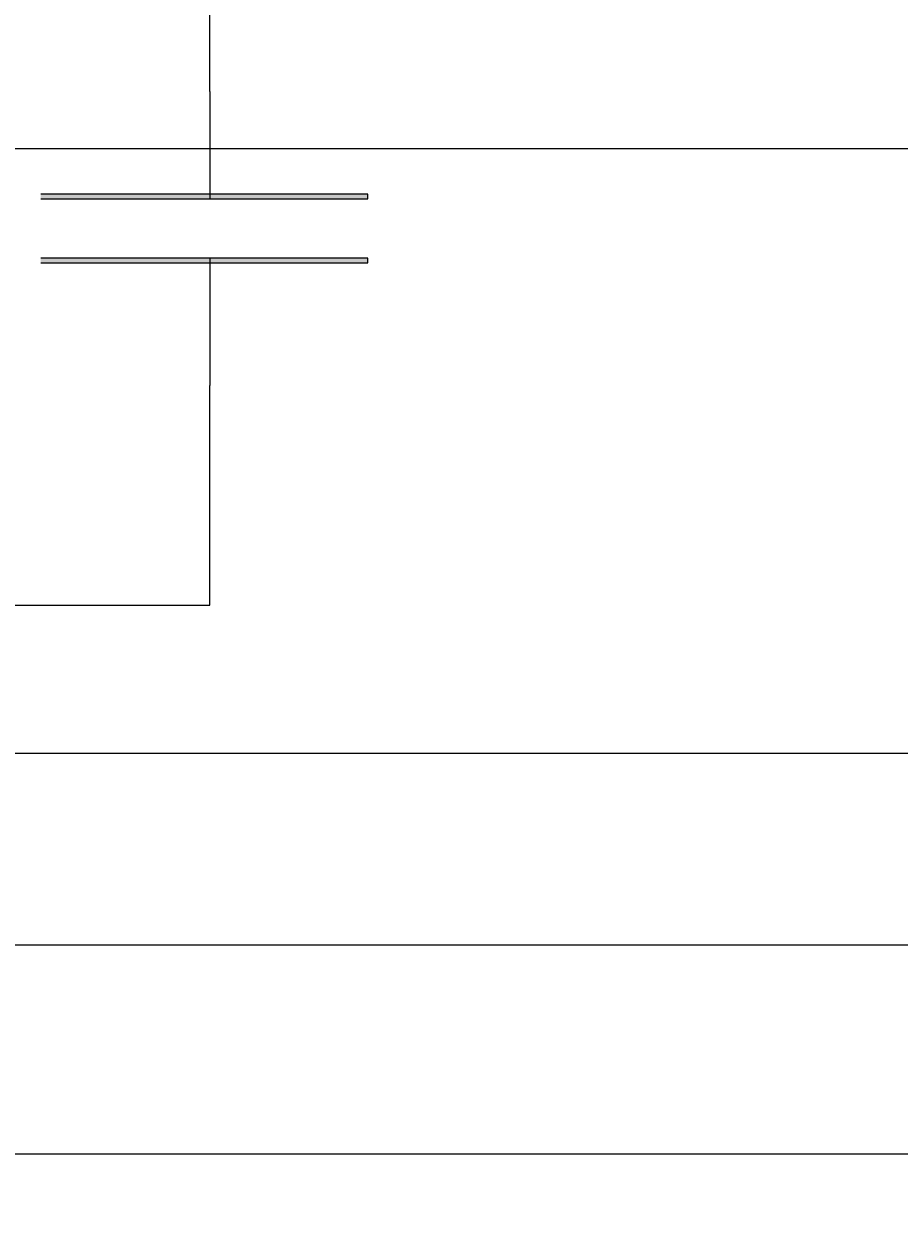
# Model space of a CAD drawing. Units: inches. Extents: x 35362 to 73946, y 43607 to 67532.
# Tile 134 of 134: x 69277 to 71350, y 55752 to 58575. Entities that reach past the tile are written whole.
import ezdxf

# ---------------------------------------------------------------- set-up
doc = ezdxf.new("R2010")
doc.units = ezdxf.units.IN
doc.header["$MEASUREMENT"] = 0
for name, color, linetype, lineweight in [('A-ANNO-DIMS', 2, 'Continuous', 18), ('E-SYMB', 1, 'Continuous', 25), ('E-SYMB-PATT', 1, 'Continuous', 13), ('E-WIRE', 3, 'Continuous', 25)]:
    doc.layers.add(name, color=color, linetype=linetype, lineweight=lineweight)
doc.styles.get("Standard").update_dxf_attribs({"font": 'arial.ttf'})
doc.dimstyles.get("Standard").update_dxf_attribs({"dimtxt": 0.18, "dimasz": 0.18, "dimexe": 0.18, "dimexo": 0.0625, "dimgap": 0.09, "dimtad": 0, "dimtih": 1, "dimtoh": 1, "dimdec": 4, "dimzin": 0, "dimdsep": 46, "dimtxsty": 'Standard', "dimcen": 0.09, "dimadec": 0, "dimazin": 0, "dimtfac": 1, "dimtdec": 4, "dimtofl": 0, "dimtmove": 0, "dimatfit": 3, "dimfxl": 1, "dimtolj": 1, "dimtzin": 0, "dimarcsym": 0})

# ---------------------------------------------------------------- blocks, each defined once
blk = doc.blocks.new('*D8')
at = {"layer": 'A-ANNO-DIMS', "color": 0, "lineweight": -2, "transparency": 16777216}
for p, q in [((66271.28651900003, 65771.51172800003), (73945.82566600003, 65771.51172800003)), ((73945.64566600005, 65771.33172800003), (73945.64566600005, 59737.03093663782)), ((73945.64566600005, 53702.36633900002), (73945.64566600005, 59736.66713036224)), ((72185.70816600003, 53702.18633900003), (73945.82566600003, 53702.18633900003))]:
    blk.add_line(p, q, dxfattribs=at)
at = {"layer": 'A-ANNO-DIMS', "color": 0, "transparency": 16777216}
for points in [[(73945.61566600006, 65771.33172800003), (73945.67566600005, 65771.33172800003), (73945.64566600005, 65771.51172800003)], [(73945.61566600006, 53702.36633900002), (73945.67566600005, 53702.36633900002), (73945.64566600005, 53702.18633900003)]]:
    blk.add_solid(points, dxfattribs=at)
at = {"layer": 'Defpoints', "color": 0, "transparency": 16777216}
for p in [(66271.22401900003, 65771.51172800003), (73945.64566600005, 65771.51172800003), (72185.64566600003, 53702.18633900003)]:
    blk.add_point(p, dxfattribs=at)
at = {"layer": 'A-ANNO-DIMS', "color": 0, "transparency": 16777216, "insert": (73945.64566600005, 59736.84903349999), "char_height": 0.18, "attachment_point": 5}
blk.add_mtext('\\A1;12069', dxfattribs=at)
blk = doc.blocks.new('*D10')
at = {"layer": 'A-ANNO-DIMS', "color": 0, "lineweight": -2, "transparency": 16777216}
for p, q in [((61240.96983600002, 59185.14395700003), (73945.82566600003, 59185.14395700003)), ((73945.64566600005, 59184.96395700003), (73945.64566600005, 56268.51827402935)), ((73945.64566600005, 53351.70866200003), (73945.64566600005, 56268.1543449707)), ((61240.96983600002, 53351.52866200003), (73945.82566600003, 53351.52866200003))]:
    blk.add_line(p, q, dxfattribs=at)
at = {"layer": 'A-ANNO-DIMS', "color": 0, "transparency": 16777216}
for points in [[(73945.61566600006, 59184.96395700003), (73945.67566600005, 59184.96395700003), (73945.64566600005, 59185.14395700003)], [(73945.61566600006, 53351.70866200003), (73945.67566600005, 53351.70866200003), (73945.64566600005, 53351.52866200003)]]:
    blk.add_solid(points, dxfattribs=at)
at = {"layer": 'Defpoints', "color": 0, "transparency": 16777216}
for p in [(61240.90733600002, 59185.14395700003), (61240.90733600002, 53351.52866200003), (73945.64566600005, 53351.52866200003)]:
    blk.add_point(p, dxfattribs=at)
at = {"layer": 'A-ANNO-DIMS', "color": 0, "transparency": 16777216, "insert": (73945.64566600005, 56268.33630949999), "char_height": 0.18, "attachment_point": 5}
blk.add_mtext('\\A1;5834', dxfattribs=at)
blk = doc.blocks.new('*D47')
at = {"layer": 'A-ANNO-DIMS', "color": 0, "lineweight": -2, "transparency": 16777216}
for p, q in [((50339.58680000003, 58279.98849500002), (73945.82566600003, 58279.98849500002)), ((73945.64566600005, 58279.80849500002), (73945.64566600005, 57564.17141502935)), ((73945.64566600005, 56848.17040600003), (73945.64566600005, 57563.80748597069)), ((50339.58680000003, 56847.99040600003), (73945.82566600003, 56847.99040600003))]:
    blk.add_line(p, q, dxfattribs=at)
at = {"layer": 'A-ANNO-DIMS', "color": 0, "transparency": 16777216}
for points in [[(73945.61566600006, 58279.80849500002), (73945.67566600005, 58279.80849500002), (73945.64566600005, 58279.98849500002)], [(73945.61566600006, 56848.17040600003), (73945.67566600005, 56848.17040600003), (73945.64566600005, 56847.99040600003)]]:
    blk.add_solid(points, dxfattribs=at)
at = {"layer": 'Defpoints', "color": 0, "transparency": 16777216}
for p in [(50339.52430000002, 58279.98849500002), (50339.52430000002, 56847.99040600003), (73945.64566600005, 56847.99040600003)]:
    blk.add_point(p, dxfattribs=at)
at = {"layer": 'A-ANNO-DIMS', "color": 0, "transparency": 16777216, "insert": (73945.64566600005, 57563.98945049999), "char_height": 0.18, "attachment_point": 5}
blk.add_mtext('\\A1;1432.0', dxfattribs=at)
blk = doc.blocks.new('*D50')
at = {"layer": 'A-ANNO-DIMS', "color": 0, "lineweight": -2, "transparency": 16777216}
for p, q in [((61657.28213900003, 56394.41825000003), (73945.82566600003, 56394.41825000003)), ((73945.64566600005, 56394.23825000003), (73945.64566600005, 56147.19337413782)), ((73945.64566600005, 55899.78469200003), (73945.64566600005, 56146.82956786224)), ((61657.28213900003, 55899.60469200002), (73945.82566600003, 55899.60469200002))]:
    blk.add_line(p, q, dxfattribs=at)
at = {"layer": 'A-ANNO-DIMS', "color": 0, "transparency": 16777216}
for points in [[(73945.61566600006, 56394.23825000003), (73945.67566600005, 56394.23825000003), (73945.64566600005, 56394.41825000003)], [(73945.61566600006, 55899.78469200003), (73945.67566600005, 55899.78469200003), (73945.64566600005, 55899.60469200002)]]:
    blk.add_solid(points, dxfattribs=at)
at = {"layer": 'Defpoints', "color": 0, "transparency": 16777216}
for p in [(61657.21963900003, 56394.41825000003), (61657.21963900003, 55899.60469200002), (73945.64566600005, 55899.60469200002)]:
    blk.add_point(p, dxfattribs=at)
at = {"layer": 'A-ANNO-DIMS', "color": 0, "transparency": 16777216, "insert": (73945.64566600005, 56147.01147099999), "char_height": 0.18, "attachment_point": 5}
blk.add_mtext('\\A1;494.8', dxfattribs=at)

msp = doc.modelspace()

# ---------------------------------------------------------------- hatches: boundary and pattern name
at = {"layer": 'E-SYMB-PATT'}
h = msp.add_hatch(color=256, dxfattribs=at)
h.dxf.hatch_style = 1
h.paths.add_polyline_path([(70091.40622432147, 58160.31058347617), (70091.40622432147, 58171.46529320917), (69317.27150299007, 58171.46529320917), (69317.27150299007, 58160.31058347618)])
h = msp.add_hatch(color=256, dxfattribs=at)
h.dxf.hatch_style = 1
h.paths.add_polyline_path([(70091.40622432147, 58009.34910605), (70091.40622432147, 58020.50381578299), (69317.27150299007, 58020.50381578299), (69317.27150299007, 58009.34910605)])

# ---------------------------------------------------------------- linework, layer by layer
at = {"layer": 'E-SYMB'}
for p, q in [((69717.45127656072, 58414.54422497431), (69717.45127656074, 58160.31058347618)), ((70091.40622432147, 58171.46529320917), (69317.27150299007, 58171.46529320917)), ((69317.27150299007, 58160.31058347618), (70091.40622432147, 58160.31058347617)), ((70091.40622432147, 58160.31058347617), (70091.40622432147, 58171.46529320917)), ((70091.40622432147, 58020.50381578299), (69317.27150299007, 58020.50381578299)), ((69717.45127656074, 58020.50381578299), (69717.45127656072, 57718.9486764754)), ((70091.40622432147, 58009.34910605), (70091.40622432147, 58020.50381578299)), ((69317.27150299007, 58009.34910605), (70091.40622432147, 58009.34910605))]:
    msp.add_line(p, q, dxfattribs=at)
at = {"layer": 'E-WIRE'}
for p, q in [((69717.45127656072, 58414.54422497431), (69717.45127656072, 58648.13900443873)), ((69717.45127656069, 57198.49827444748), (69717.45127656072, 57718.9486764754)), ((68678.61631230469, 57198.49827444747), (69717.45127656069, 57198.49827444748))]:
    msp.add_line(p, q, dxfattribs=at)

# ---------------------------------------------------------------- dimensions: what is measured, and where the dimension line sits
at = {"layer": 'A-ANNO-DIMS'}
for base, p1, p2, override, picture, middle in [((73945.64566600005, 65771.51172800003), (72185.645666, 53702.186339), (66271.224019, 65771.51172799998), {"dimdec": 0, "dimlfac": 1, "dimrnd": 0, "dimzin": 0, "dimdsep": 46, "dimlunit": 2}, '*D8', (73945.64566600005, 59736.84903349999)), ((73945.64566600005, 53351.52866200003), (61240.907336, 59185.14395699999), (61240.907336, 53351.52866199999), {"dimdec": 0, "dimlfac": 1, "dimrnd": 0, "dimzin": 0, "dimdsep": 46, "dimlunit": 2}, '*D10', (73945.64566600005, 56268.33630949999)), ((73945.64566600005, 56847.99040600003), (50339.5243, 58279.988495), (50339.5243, 56847.99040599999), {"dimdec": 1, "dimlfac": 1, "dimrnd": 0, "dimzin": 0, "dimdsep": 46, "dimlunit": 2}, '*D47', (73945.64566600005, 57563.98945049999)), ((73945.64566600005, 55899.60469200002), (61657.219639, 56394.41825), (61657.219639, 55899.604692), {"dimdec": 1, "dimlfac": 1, "dimrnd": 0, "dimzin": 0, "dimdsep": 46, "dimlunit": 2}, '*D50', (73945.64566600005, 56147.01147099999))]:
    dim = msp.add_linear_dim(base=base, p1=p1, p2=p2, angle=90, dimstyle='Standard', override=override, dxfattribs=at)
    dim.commit()
    dim.dimension.update_dxf_attribs({"geometry": picture, "text_midpoint": middle})

doc.saveas('drawing.dxf')
